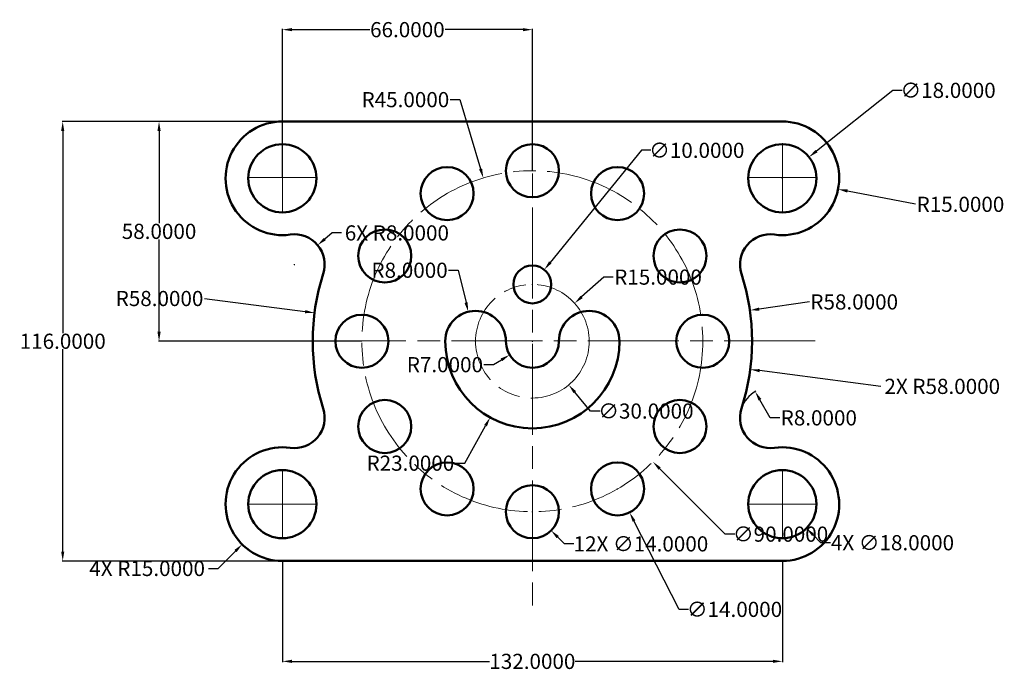
# Model space of a CAD drawing. Units: inches. Extents: x 631 to 891, y 582 to 754.
import ezdxf

# ---------------------------------------------------------------- set-up
doc = ezdxf.new("R2010")
doc.units = ezdxf.units.IN
doc.header["$MEASUREMENT"] = 0
doc.linetypes.add('ACAD_ISO08W100', pattern=[36, 24, -3, 6, -3])
for name, color, linetype, lineweight in [('M-CNTR', 4, 'ACAD_ISO08W100', 18), ('M-CNTR-MARK', 4, 'Continuous', 18), ('M-DIMS', 2, 'Continuous', 25), ('M-OUTL', 7, 'Continuous', 50)]:
    doc.layers.add(name, color=color, linetype=linetype, lineweight=lineweight)
doc.styles.get("Standard").update_dxf_attribs({"font": 'arial.ttf'})
doc.dimstyles.get("Standard").update_dxf_attribs({"dimtxt": 4, "dimasz": 2.5, "dimexe": 0.18, "dimexo": 0.0625, "dimgap": 0.09, "dimtad": 0, "dimtih": 1, "dimtoh": 1, "dimdec": 4, "dimzin": 0, "dimdsep": 46, "dimtxsty": 'Standard', "dimcen": 0.09, "dimadec": 0, "dimazin": 0, "dimtfac": 1, "dimtdec": 4, "dimtofl": 0, "dimtmove": 0, "dimatfit": 3, "dimfxl": 1, "dimtolj": 1, "dimtzin": 0, "dimarcsym": 0})

# ---------------------------------------------------------------- blocks, each defined once
blk = doc.blocks.new('*D1')
at = {"layer": 'Defpoints', "color": 0, "lineweight": 100, "transparency": 16777216}
for p in [(777.54, 678.87), (766.39, 668.84)]:
    blk.add_point(p, dxfattribs=at)
at = {"layer": 'M-DIMS', "color": 0, "lineweight": -2, "transparency": 16777216}
for p, q in [((785.22, 685.77), (779.4, 680.54)), ((787.72, 685.77), (785.22, 685.77)), ((766.3, 668.84), (766.48, 668.84)), ((766.39, 668.75), (766.39, 668.93))]:
    blk.add_line(p, q, dxfattribs=at)
at = {"layer": 'M-DIMS', "color": 0, "lineweight": 100, "transparency": 16777216}
blk.add_solid([(779.13, 680.85), (779.68, 680.23), (777.54, 678.87)], dxfattribs=at)
at = {"layer": 'M-DIMS', "color": 0, "transparency": 16777216, "insert": (799.57, 685.77), "char_height": 4, "attachment_point": 5}
blk.add_mtext('\\A1;R15.0000', dxfattribs=at)
blk = doc.blocks.new('*D2')
at = {"layer": 'Defpoints', "color": 0, "lineweight": 100, "transparency": 16777216}
for p in [(708.87, 676.33), (766.39, 668.84)]:
    blk.add_point(p, dxfattribs=at)
at = {"layer": 'M-DIMS', "color": 0, "lineweight": -2, "transparency": 16777216}
for p, q in [((679.82, 680.12), (706.39, 676.66)), ((766.3, 668.84), (766.48, 668.84)), ((766.39, 668.75), (766.39, 668.93))]:
    blk.add_line(p, q, dxfattribs=at)
at = {"layer": 'M-DIMS', "color": 0, "lineweight": 100, "transparency": 16777216}
blk.add_solid([(706.45, 677.07), (706.34, 676.24), (708.87, 676.33)], dxfattribs=at)
at = {"layer": 'M-DIMS', "color": 0, "transparency": 16777216, "insert": (667.96, 680.12), "char_height": 4, "attachment_point": 5}
blk.add_mtext('\\A1;R58.0000', dxfattribs=at)
blk = doc.blocks.new('*D3')
at = {"layer": 'Defpoints', "color": 0, "lineweight": 100, "transparency": 16777216}
for p in [(823.81, 676.99), (766.39, 668.84)]:
    blk.add_point(p, dxfattribs=at)
at = {"layer": 'M-DIMS', "color": 0, "lineweight": -2, "transparency": 16777216}
for p, q in [((839.51, 679.22), (826.29, 677.34)), ((766.3, 668.84), (766.48, 668.84)), ((766.39, 668.75), (766.39, 668.93))]:
    blk.add_line(p, q, dxfattribs=at)
at = {"layer": 'M-DIMS', "color": 0, "lineweight": 100, "transparency": 16777216}
blk.add_solid([(826.23, 677.75), (826.35, 676.93), (823.81, 676.99)], dxfattribs=at)
at = {"layer": 'M-DIMS', "color": 0, "transparency": 16777216, "insert": (851.36, 679.22), "char_height": 4, "attachment_point": 5}
blk.add_mtext('\\A1;R58.0000', dxfattribs=at)
blk = doc.blocks.new('*D4')
at = {"layer": 'Defpoints', "color": 0, "lineweight": 100, "transparency": 16777216}
for p in [(832.39, 711.84), (847.11, 708.97)]:
    blk.add_point(p, dxfattribs=at)
at = {"layer": 'M-DIMS', "color": 0, "lineweight": -2, "transparency": 16777216}
for p, q in [((832.3, 711.84), (832.48, 711.84)), ((832.39, 711.75), (832.39, 711.93)), ((867.55, 704.98), (849.56, 708.49))]:
    blk.add_line(p, q, dxfattribs=at)
at = {"layer": 'M-DIMS', "color": 0, "lineweight": 100, "transparency": 16777216}
blk.add_solid([(849.64, 708.9), (849.48, 708.08), (847.11, 708.97)], dxfattribs=at)
at = {"layer": 'M-DIMS', "color": 0, "transparency": 16777216, "insert": (879.41, 704.98), "char_height": 4, "attachment_point": 5}
blk.add_mtext('\\A1;R15.0000', dxfattribs=at)
blk = doc.blocks.new('*D5')
at = {"layer": 'Defpoints', "color": 0, "lineweight": 100, "transparency": 16777216}
for p in [(825.21, 655.55), (829.21, 648.62)]:
    blk.add_point(p, dxfattribs=at)
at = {"layer": 'M-DIMS', "color": 0, "lineweight": -2, "transparency": 16777216}
for p, q in [((829.21, 648.62), (826.46, 653.39)), ((831.71, 648.62), (829.21, 648.62))]:
    blk.add_line(p, q, dxfattribs=at)
blk.add_arc((829.21, 648.62), 8, 118.7108, 161.7121, dxfattribs=at)
at = {"layer": 'M-DIMS', "color": 0, "lineweight": 100, "transparency": 16777216}
blk.add_solid([(826.83, 653.6), (826.1, 653.18), (825.21, 655.55)], dxfattribs=at)
at = {"layer": 'M-DIMS', "color": 0, "transparency": 16777216, "insert": (842.01, 648.62), "char_height": 4, "attachment_point": 5}
blk.add_mtext('\\A1;R8.0000', dxfattribs=at)
blk = doc.blocks.new('*D6')
at = {"layer": 'Defpoints', "color": 0, "lineweight": 100, "transparency": 16777216}
for p in [(749.47, 676.61), (751.39, 668.84)]:
    blk.add_point(p, dxfattribs=at)
at = {"layer": 'M-DIMS', "color": 0, "lineweight": -2, "transparency": 16777216}
for p, q in [((744.27, 687.58), (746.77, 687.58)), ((746.77, 687.58), (748.87, 679.04)), ((751.3, 668.84), (751.48, 668.84)), ((751.39, 668.75), (751.39, 668.93))]:
    blk.add_line(p, q, dxfattribs=at)
at = {"layer": 'M-DIMS', "color": 0, "lineweight": 100, "transparency": 16777216}
blk.add_solid([(749.28, 679.14), (748.47, 678.94), (749.47, 676.61)], dxfattribs=at)
at = {"layer": 'M-DIMS', "color": 0, "transparency": 16777216, "insert": (733.97, 687.58), "char_height": 4, "attachment_point": 5}
blk.add_mtext('\\A1;R8.0000', dxfattribs=at)
blk = doc.blocks.new('*D7')
at = {"layer": 'Defpoints', "color": 0, "lineweight": 100, "transparency": 16777216}
for p in [(753.44, 711.94), (766.39, 668.84)]:
    blk.add_point(p, dxfattribs=at)
at = {"layer": 'M-DIMS', "color": 0, "lineweight": -2, "transparency": 16777216}
for p, q in [((744.73, 732.61), (747.23, 732.61)), ((747.23, 732.61), (752.72, 714.33)), ((766.3, 668.84), (766.48, 668.84)), ((766.39, 668.75), (766.39, 668.93))]:
    blk.add_line(p, q, dxfattribs=at)
at = {"layer": 'M-DIMS', "color": 0, "lineweight": 100, "transparency": 16777216}
blk.add_solid([(753.12, 714.45), (752.32, 714.21), (753.44, 711.94)], dxfattribs=at)
at = {"layer": 'M-DIMS', "color": 0, "transparency": 16777216, "insert": (732.87, 732.61), "char_height": 4, "attachment_point": 5}
blk.add_mtext('\\A1;R45.0000', dxfattribs=at)
blk = doc.blocks.new('*D8')
at = {"layer": 'Defpoints', "color": 0, "lineweight": 100, "transparency": 16777216}
for p in [(785.7, 636.11), (792.07, 623.64)]:
    blk.add_point(p, dxfattribs=at)
at = {"layer": 'M-DIMS', "color": 0, "lineweight": -2, "transparency": 16777216}
for p, q in [((788.8, 629.87), (788.98, 629.87)), ((788.89, 629.78), (788.89, 629.96)), ((805.15, 598.07), (793.21, 621.41)), ((807.65, 598.07), (805.15, 598.07))]:
    blk.add_line(p, q, dxfattribs=at)
at = {"layer": 'M-DIMS', "color": 0, "lineweight": 100, "transparency": 16777216}
blk.add_solid([(793.58, 621.6), (792.84, 621.22), (792.07, 623.64)], dxfattribs=at)
at = {"layer": 'M-DIMS', "color": 0, "transparency": 16777216, "insert": (819.76, 598.07), "char_height": 4, "attachment_point": 5}
blk.add_mtext('\\A1;∅14.0000', dxfattribs=at)
blk = doc.blocks.new('*D9')
at = {"layer": 'Defpoints', "color": 0, "lineweight": 100, "transparency": 16777216}
for p in [(769.54, 687.72), (763.23, 679.97)]:
    blk.add_point(p, dxfattribs=at)
at = {"layer": 'M-DIMS', "color": 0, "lineweight": -2, "transparency": 16777216}
for p, q in [((795.19, 719.23), (771.12, 689.66)), ((797.69, 719.23), (795.19, 719.23)), ((766.3, 683.84), (766.48, 683.84)), ((766.39, 683.75), (766.39, 683.93))]:
    blk.add_line(p, q, dxfattribs=at)
at = {"layer": 'M-DIMS', "color": 0, "lineweight": 100, "transparency": 16777216}
blk.add_solid([(770.8, 689.92), (771.45, 689.4), (769.54, 687.72)], dxfattribs=at)
at = {"layer": 'M-DIMS', "color": 0, "transparency": 16777216, "insert": (809.8, 719.23), "char_height": 4, "attachment_point": 5}
blk.add_mtext('\\A1;∅10.0000', dxfattribs=at)
blk = doc.blocks.new('*D10')
at = {"layer": 'Defpoints', "color": 0, "lineweight": 100, "transparency": 16777216}
for p in [(700.39, 610.84), (832.39, 610.84), (832.39, 584.35)]:
    blk.add_point(p, dxfattribs=at)
at = {"layer": 'M-DIMS', "color": 0, "lineweight": -2, "transparency": 16777216}
for p, q in [((700.39, 610.78), (700.39, 584.17)), ((832.39, 610.78), (832.39, 584.17)), ((702.89, 584.35), (755.08, 584.35)), ((829.89, 584.35), (777.69, 584.35))]:
    blk.add_line(p, q, dxfattribs=at)
at = {"layer": 'M-DIMS', "color": 0, "lineweight": 100, "transparency": 16777216}
for points in [[(702.89, 584.77), (702.89, 583.94), (700.39, 584.35)], [(829.89, 584.77), (829.89, 583.94), (832.39, 584.35)]]:
    blk.add_solid(points, dxfattribs=at)
at = {"layer": 'M-DIMS', "color": 0, "transparency": 16777216, "insert": (766.39, 584.35), "char_height": 4, "attachment_point": 5}
blk.add_mtext('\\A1;132.0000', dxfattribs=at)
blk = doc.blocks.new('*D11')
at = {"layer": 'Defpoints', "color": 0, "lineweight": 100, "transparency": 16777216}
for p in [(642.4, 726.84), (700.39, 726.84), (700.39, 610.84)]:
    blk.add_point(p, dxfattribs=at)
at = {"layer": 'M-DIMS', "color": 0, "lineweight": -2, "transparency": 16777216}
for p, q in [((700.33, 726.84), (642.22, 726.84)), ((642.4, 724.34), (642.4, 670.98)), ((642.4, 613.34), (642.4, 666.71)), ((700.33, 610.84), (642.22, 610.84))]:
    blk.add_line(p, q, dxfattribs=at)
at = {"layer": 'M-DIMS', "color": 0, "lineweight": 100, "transparency": 16777216}
for points in [[(641.98, 724.34), (642.81, 724.34), (642.4, 726.84)], [(641.98, 613.34), (642.81, 613.34), (642.4, 610.84)]]:
    blk.add_solid(points, dxfattribs=at)
at = {"layer": 'M-DIMS', "color": 0, "transparency": 16777216, "insert": (642.4, 668.84), "char_height": 4, "attachment_point": 5}
blk.add_mtext('\\A1;116.0000', dxfattribs=at)
blk = doc.blocks.new('*D12')
at = {"layer": 'Defpoints', "color": 0, "lineweight": 100, "transparency": 16777216}
for p in [(667.83, 726.84), (721.39, 726.84), (721.39, 668.84)]:
    blk.add_point(p, dxfattribs=at)
at = {"layer": 'M-DIMS', "color": 0, "lineweight": -2, "transparency": 16777216}
for p, q in [((721.33, 726.84), (667.65, 726.84)), ((667.83, 724.34), (667.83, 699.98)), ((667.83, 671.34), (667.83, 695.71)), ((721.33, 668.84), (667.65, 668.84))]:
    blk.add_line(p, q, dxfattribs=at)
at = {"layer": 'M-DIMS', "color": 0, "lineweight": 100, "transparency": 16777216}
for points in [[(667.41, 724.34), (668.25, 724.34), (667.83, 726.84)], [(667.41, 671.34), (668.25, 671.34), (667.83, 668.84)]]:
    blk.add_solid(points, dxfattribs=at)
at = {"layer": 'M-DIMS', "color": 0, "transparency": 16777216, "insert": (667.83, 697.84), "char_height": 4, "attachment_point": 5}
blk.add_mtext('\\A1;58.0000', dxfattribs=at)
blk = doc.blocks.new('*D13')
at = {"layer": 'Defpoints', "color": 0, "lineweight": 100, "transparency": 16777216}
for p in [(766.39, 751.08), (766.39, 713.84), (700.39, 712.08)]:
    blk.add_point(p, dxfattribs=at)
at = {"layer": 'M-DIMS', "color": 0, "lineweight": -2, "transparency": 16777216}
for p, q in [((700.39, 712.14), (700.39, 751.26)), ((766.39, 713.91), (766.39, 751.26)), ((702.89, 751.08), (723.44, 751.08)), ((763.89, 751.08), (743.34, 751.08))]:
    blk.add_line(p, q, dxfattribs=at)
at = {"layer": 'M-DIMS', "color": 0, "lineweight": 100, "transparency": 16777216}
for points in [[(702.89, 751.5), (702.89, 750.67), (700.39, 751.08)], [(763.89, 751.5), (763.89, 750.67), (766.39, 751.08)]]:
    blk.add_solid(points, dxfattribs=at)
at = {"layer": 'M-DIMS', "color": 0, "transparency": 16777216, "insert": (733.39, 751.08), "char_height": 4, "attachment_point": 5}
blk.add_mtext('\\A1;66.0000', dxfattribs=at)
blk = doc.blocks.new('*D14')
at = {"layer": 'Defpoints', "color": 0, "lineweight": 100, "transparency": 16777216}
for p in [(839.43, 717.45), (825.35, 706.23)]:
    blk.add_point(p, dxfattribs=at)
at = {"layer": 'M-DIMS', "color": 0, "lineweight": -2, "transparency": 16777216}
for p, q in [((861.52, 735.06), (841.38, 719.01)), ((864.02, 735.06), (861.52, 735.06)), ((832.3, 711.84), (832.48, 711.84)), ((832.39, 711.75), (832.39, 711.93))]:
    blk.add_line(p, q, dxfattribs=at)
at = {"layer": 'M-DIMS', "color": 0, "lineweight": 100, "transparency": 16777216}
blk.add_solid([(841.12, 719.34), (841.64, 718.69), (839.43, 717.45)], dxfattribs=at)
at = {"layer": 'M-DIMS', "color": 0, "transparency": 16777216, "insert": (876.14, 735.06), "char_height": 4, "attachment_point": 5}
blk.add_mtext('\\A1;∅18.0000', dxfattribs=at)
blk = doc.blocks.new('MOUNT-HOLE-D18')
blk.add_circle((0, 0), 9)
blk = doc.blocks.new('BOLT-CIRCLE-HOLE-D14')
blk.add_circle((0, 0), 7)
blk = doc.blocks.new('CENTER-MARK-D18')
for p, q in [((0, 9), (0, -9)), ((0, 0), (-9, 0)), ((0, 0), (9, 0))]:
    blk.add_line(p, q)
blk = doc.blocks.new('*D18')
at = {"layer": 'Defpoints', "color": 0, "lineweight": 100, "transparency": 16777216}
for p in [(700.39, 625.84), (689.78, 615.24)]:
    blk.add_point(p, dxfattribs=at)
at = {"layer": 'M-DIMS', "color": 0, "lineweight": -2, "transparency": 16777216}
for p, q in [((700.3, 625.84), (700.48, 625.84)), ((700.39, 625.75), (700.39, 625.93)), ((683.42, 608.87), (688.01, 613.47)), ((680.92, 608.87), (683.42, 608.87))]:
    blk.add_line(p, q, dxfattribs=at)
at = {"layer": 'M-DIMS', "color": 0, "lineweight": 100, "transparency": 16777216}
blk.add_solid([(687.72, 613.76), (688.31, 613.18), (689.78, 615.24)], dxfattribs=at)
at = {"layer": 'M-DIMS', "color": 0, "transparency": 16777216, "insert": (664.69, 608.87), "char_height": 4, "attachment_point": 5}
blk.add_mtext('\\A1;4X R15.0000', dxfattribs=at)
blk = doc.blocks.new('*D19')
at = {"layer": 'Defpoints', "color": 0, "lineweight": 100, "transparency": 16777216}
for p in [(766.39, 668.84), (823.91, 661.4)]:
    blk.add_point(p, dxfattribs=at)
at = {"layer": 'M-DIMS', "color": 0, "lineweight": -2, "transparency": 16777216}
for p, q in [((766.3, 668.84), (766.48, 668.84)), ((766.39, 668.75), (766.39, 668.93)), ((858.42, 656.93), (826.39, 661.08))]:
    blk.add_line(p, q, dxfattribs=at)
at = {"layer": 'M-DIMS', "color": 0, "lineweight": 100, "transparency": 16777216}
blk.add_solid([(826.44, 661.49), (826.33, 660.66), (823.91, 661.4)], dxfattribs=at)
at = {"layer": 'M-DIMS', "color": 0, "transparency": 16777216, "insert": (874.61, 656.93), "char_height": 4, "attachment_point": 5}
blk.add_mtext('\\A1;2X R58.0000', dxfattribs=at)
blk = doc.blocks.new('*D20')
at = {"layer": 'Defpoints', "color": 0, "lineweight": 100, "transparency": 16777216}
for p in [(709.69, 694.21), (703.56, 689.06)]:
    blk.add_point(p, dxfattribs=at)
at = {"layer": 'M-DIMS', "color": 0, "lineweight": -2, "transparency": 16777216}
for p, q in [((713.51, 697.43), (711.6, 695.82)), ((716.01, 697.43), (713.51, 697.43)), ((703.47, 689.06), (703.65, 689.06)), ((703.56, 688.97), (703.56, 689.15))]:
    blk.add_line(p, q, dxfattribs=at)
at = {"layer": 'M-DIMS', "color": 0, "lineweight": 100, "transparency": 16777216}
blk.add_solid([(711.33, 696.14), (711.87, 695.5), (709.69, 694.21)], dxfattribs=at)
at = {"layer": 'M-DIMS', "color": 0, "transparency": 16777216, "insert": (730.62, 697.43), "char_height": 4, "attachment_point": 5}
blk.add_mtext('\\A1;6X R8.0000', dxfattribs=at)
blk = doc.blocks.new('*D21')
at = {"layer": 'Defpoints', "color": 0, "lineweight": 100, "transparency": 16777216}
for p in [(734.57, 700.66), (798.21, 637.02)]:
    blk.add_point(p, dxfattribs=at)
at = {"layer": 'M-DIMS', "color": 0, "lineweight": -2, "transparency": 16777216}
for p, q in [((766.3, 668.84), (766.48, 668.84)), ((766.39, 668.75), (766.39, 668.93)), ((817.3, 617.93), (799.98, 635.26)), ((819.8, 617.93), (817.3, 617.93))]:
    blk.add_line(p, q, dxfattribs=at)
at = {"layer": 'M-DIMS', "color": 0, "lineweight": 100, "transparency": 16777216}
blk.add_solid([(800.27, 635.55), (799.68, 634.96), (798.21, 637.02)], dxfattribs=at)
at = {"layer": 'M-DIMS', "color": 0, "transparency": 16777216, "insert": (831.92, 617.93), "char_height": 4, "attachment_point": 5}
blk.add_mtext('\\A1;∅90.0000', dxfattribs=at)
blk = doc.blocks.new('*D22')
at = {"layer": 'Defpoints', "color": 0, "lineweight": 100, "transparency": 16777216}
for p in [(826.02, 632.21), (838.75, 619.48)]:
    blk.add_point(p, dxfattribs=at)
at = {"layer": 'M-DIMS', "color": 0, "lineweight": -2, "transparency": 16777216}
for p, q in [((832.3, 625.84), (832.48, 625.84)), ((832.39, 625.75), (832.39, 625.93)), ((842.57, 615.66), (840.52, 617.71)), ((845.07, 615.66), (842.57, 615.66))]:
    blk.add_line(p, q, dxfattribs=at)
at = {"layer": 'M-DIMS', "color": 0, "lineweight": 100, "transparency": 16777216}
blk.add_solid([(840.81, 618.01), (840.23, 617.42), (838.75, 619.48)], dxfattribs=at)
at = {"layer": 'M-DIMS', "color": 0, "transparency": 16777216, "insert": (861.46, 615.66), "char_height": 4, "attachment_point": 5}
blk.add_mtext('\\A1;4X ∅18.0000', dxfattribs=at)
blk = doc.blocks.new('*D23')
at = {"layer": 'Defpoints', "color": 0, "lineweight": 100, "transparency": 16777216}
for p in [(761.44, 628.79), (771.34, 618.89)]:
    blk.add_point(p, dxfattribs=at)
at = {"layer": 'M-DIMS', "color": 0, "lineweight": -2, "transparency": 16777216}
for p, q in [((766.39, 623.75), (766.39, 623.93)), ((766.3, 623.84), (766.48, 623.84)), ((774.87, 615.36), (773.11, 617.13)), ((777.37, 615.36), (774.87, 615.36))]:
    blk.add_line(p, q, dxfattribs=at)
at = {"layer": 'M-DIMS', "color": 0, "lineweight": 100, "transparency": 16777216}
blk.add_solid([(773.4, 617.42), (772.81, 616.83), (771.34, 618.89)], dxfattribs=at)
at = {"layer": 'M-DIMS', "color": 0, "transparency": 16777216, "insert": (795.05, 615.36), "char_height": 4, "attachment_point": 5}
blk.add_mtext('\\A1;12X ∅14.0000', dxfattribs=at)
blk = doc.blocks.new('*D24')
at = {"layer": 'Defpoints', "color": 0, "lineweight": 100, "transparency": 16777216}
for p in [(766.39, 668.84), (755.24, 648.73)]:
    blk.add_point(p, dxfattribs=at)
at = {"layer": 'M-DIMS', "color": 0, "lineweight": -2, "transparency": 16777216}
for p, q in [((766.3, 668.84), (766.48, 668.84)), ((766.39, 668.75), (766.39, 668.93)), ((748.55, 636.66), (754.03, 646.54)), ((746.05, 636.66), (748.55, 636.66))]:
    blk.add_line(p, q, dxfattribs=at)
at = {"layer": 'M-DIMS', "color": 0, "lineweight": 100, "transparency": 16777216}
blk.add_solid([(753.66, 646.74), (754.39, 646.34), (755.24, 648.73)], dxfattribs=at)
at = {"layer": 'M-DIMS', "color": 0, "transparency": 16777216, "insert": (734.19, 636.66), "char_height": 4, "attachment_point": 5}
blk.add_mtext('\\A1;R23.0000', dxfattribs=at)
blk = doc.blocks.new('*D25')
at = {"layer": 'Defpoints', "color": 0, "lineweight": 100, "transparency": 16777216}
for p in [(766.39, 668.84), (760.39, 665.24)]:
    blk.add_point(p, dxfattribs=at)
at = {"layer": 'M-DIMS', "color": 0, "lineweight": -2, "transparency": 16777216}
for p, q in [((766.3, 668.84), (766.48, 668.84)), ((766.39, 668.75), (766.39, 668.93)), ((756.1, 662.66), (758.25, 663.95)), ((753.6, 662.66), (756.1, 662.66))]:
    blk.add_line(p, q, dxfattribs=at)
at = {"layer": 'M-DIMS', "color": 0, "lineweight": 100, "transparency": 16777216}
blk.add_solid([(758.03, 664.31), (758.46, 663.59), (760.39, 665.24)], dxfattribs=at)
at = {"layer": 'M-DIMS', "color": 0, "transparency": 16777216, "insert": (743.3, 662.66), "char_height": 4, "attachment_point": 5}
blk.add_mtext('\\A1;R7.0000', dxfattribs=at)
blk = doc.blocks.new('*D26')
at = {"layer": 'Defpoints', "color": 0, "lineweight": 100, "transparency": 16777216}
for p in [(756.79, 680.37), (775.99, 657.32)]:
    blk.add_point(p, dxfattribs=at)
at = {"layer": 'M-DIMS', "color": 0, "lineweight": -2, "transparency": 16777216}
for p, q in [((766.3, 668.84), (766.48, 668.84)), ((766.39, 668.75), (766.39, 668.93)), ((781.75, 650.41), (777.59, 655.4)), ((784.25, 650.41), (781.75, 650.41))]:
    blk.add_line(p, q, dxfattribs=at)
at = {"layer": 'M-DIMS', "color": 0, "lineweight": 100, "transparency": 16777216}
blk.add_solid([(777.91, 655.67), (777.27, 655.13), (775.99, 657.32)], dxfattribs=at)
at = {"layer": 'M-DIMS', "color": 0, "transparency": 16777216, "insert": (796.37, 650.41), "char_height": 4, "attachment_point": 5}
blk.add_mtext('\\A1;∅30.0000', dxfattribs=at)

msp = doc.modelspace()

# ---------------------------------------------------------------- linework, layer by layer
at = {"layer": 'M-CNTR'}
for p, q in [((766.38827, 740.12463), (766.38827, 597.79966)), ((841.02678, 668.96214), (692.87285, 668.96214))]:
    msp.add_line(p, q, dxfattribs=at)
for radius in [45, 15]:
    msp.add_circle((766.38827, 668.84399), radius, dxfattribs=at)
at = {"layer": 'M-OUTL'}
for p, q in [((700.38827, 726.84399), (832.38827, 726.84399)), ((700.38827, 610.84399), (832.38827, 610.84399))]:
    msp.add_line(p, q, dxfattribs=at)
msp.add_circle((766.38827, 683.84399), 5, dxfattribs=at)
for centre, radius, start, end in [((700.38827, 711.84399), 15, 90, 277.9312313), ((832.38827, 711.84399), 15, 262.0687687, 90), ((703.56191, 689.064), 8, 342.1597695, 97.9312313), ((829.21463, 689.064), 8, 82.0687687, 197.8402305), ((766.38827, 668.84399), 58, 162.1597695, 197.8402305), ((766.38827, 668.84399), 58, 342.1597695, 17.8402305), ((751.38827, 668.84399), 8, 0, 180), ((781.38827, 668.84399), 8, 0, 180), ((766.38827, 668.84399), 23, 180, 0), ((766.38827, 668.84399), 7, 180, 0), ((703.56191, 648.62398), 8, 262.0687687, 17.8402305), ((829.21463, 648.62398), 8, 162.1597695, 277.9312313), ((700.38827, 625.84399), 15, 82.0687687, 270), ((832.38827, 625.84399), 15, 270, 97.9312313)]:
    msp.add_arc(centre, radius, start, end, dxfattribs=at)

# ---------------------------------------------------------------- block references
at = {"layer": 'M-CNTR-MARK'}
for p in [(700.38827, 712.08029), (832.38827, 712.08029), (832.38827, 625.84399)]:
    msp.add_blockref('CENTER-MARK-D18', p, dxfattribs=at)
at = {"layer": 'M-CNTR-MARK', "rotation": 180}
msp.add_blockref('CENTER-MARK-D18', (700.38827, 625.84399), dxfattribs=at)
at = {"layer": 'M-OUTL'}
for name, p in [('MOUNT-HOLE-D18', (700.38827, 711.84399)), ('BOLT-CIRCLE-HOLE-D14', (766.38827, 713.84399)), ('MOUNT-HOLE-D18', (832.38827, 711.84399)), ('BOLT-CIRCLE-HOLE-D14', (743.88827, 707.81514)), ('BOLT-CIRCLE-HOLE-D14', (788.88827, 707.81514)), ('BOLT-CIRCLE-HOLE-D14', (727.41713, 691.34399)), ('BOLT-CIRCLE-HOLE-D14', (805.35941, 691.34399)), ('BOLT-CIRCLE-HOLE-D14', (721.38827, 668.84399)), ('BOLT-CIRCLE-HOLE-D14', (811.38827, 668.84399)), ('BOLT-CIRCLE-HOLE-D14', (727.41713, 646.34399)), ('BOLT-CIRCLE-HOLE-D14', (805.35941, 646.34399)), ('BOLT-CIRCLE-HOLE-D14', (743.88827, 629.87285)), ('BOLT-CIRCLE-HOLE-D14', (788.88827, 629.87285)), ('MOUNT-HOLE-D18', (700.38827, 625.84399)), ('MOUNT-HOLE-D18', (832.38827, 625.84399)), ('BOLT-CIRCLE-HOLE-D14', (766.38827, 623.84399))]:
    msp.add_blockref(name, p, dxfattribs=at)

# ---------------------------------------------------------------- dimensions: what is measured, and where the dimension line sits
at = {"layer": 'M-DIMS'}
for base, p1, p2, picture, middle in [((766.38827, 751.08415), (700.38827, 712.08029), (766.38827, 713.84399), '*D13', (733.38827, 751.08415)), ((832.38827, 584.35212), (700.38827, 610.84399), (832.38827, 610.84399), '*D10', (766.38827, 584.35212))]:
    dim = msp.add_linear_dim(base=base, p1=p1, p2=p2, dimstyle='Standard', override={"dimclrd": 0, "dimclre": 0, "dimclrt": 0}, dxfattribs=at)
    dim.commit()
    dim.dimension.update_dxf_attribs({"geometry": picture, "text_midpoint": middle})
for p1, p2, override, picture, middle in [((825.34999, 706.23483), (839.42655, 717.45315), {"dimclrd": 0, "dimclre": 0, "dimclrt": 0}, '*D14', (876.13632, 735.06085)), ((763.23248, 679.96572), (769.54406, 687.72226), {"dimclrd": 0, "dimclre": 0, "dimclrt": 0}, '*D9', (809.80145, 719.23404)), ((734.5686, 700.66393), (798.20794, 637.02406), {"dimdec": 4, "dimlfac": 1, "dimrnd": 0, "dimzin": 0, "dimdsep": 46, "dimlunit": 2}, '*D21', (831.91567, 617.93209)), ((756.78645, 680.3681), (775.99009, 657.31989), {"dimdec": 4, "dimlfac": 1, "dimrnd": 0, "dimzin": 0, "dimdsep": 46, "dimlunit": 2}, '*D26', (796.36711, 650.40543)), ((785.70231, 636.1058), (792.07423, 623.6399), {"dimclrd": 0, "dimclre": 0, "dimclrt": 0}, '*D8', (819.76177, 598.06678))]:
    dim = msp.add_diameter_dim_2p(p1=p1, p2=p2, dimstyle='Standard', override=override, dxfattribs=at)
    dim.commit()
    dim.dimension.update_dxf_attribs({"geometry": picture, "text_midpoint": middle, "dimtype": 163})
for center, mpoint, override, picture, middle in [((766.38827, 668.84399), (753.43666, 711.93988), {"dimclrd": 0, "dimclre": 0, "dimclrt": 0}, '*D7', (732.87159, 732.607)), ((832.38827, 711.84399), (847.11036, 708.96994), {"dimclrd": 0, "dimclre": 0, "dimclrt": 0}, '*D4', (867.55304, 704.97911)), ((751.38827, 668.84399), (749.47252, 676.61122), {"dimclrd": 0, "dimclre": 0, "dimclrt": 0}, '*D6', (733.96763, 687.57754)), ((766.38827, 668.84399), (777.54444, 678.87095), {"dimclrd": 0, "dimclre": 0, "dimclrt": 0}, '*D1', (799.57396, 685.76958)), ((766.38827, 668.84399), (708.87405, 676.33498), {"dimclrd": 0, "dimclre": 0, "dimclrt": 0}, '*D2', (679.81556, 680.11972)), ((766.38827, 668.84399), (823.8134, 676.9898), {"dimclrd": 0, "dimclre": 0, "dimclrt": 0}, '*D3', (839.50552, 679.21575)), ((766.38827, 668.84399), (755.23849, 648.72727), {"dimdec": 4, "dimlfac": 1, "dimrnd": 0, "dimzin": 0, "dimdsep": 46, "dimlunit": 2}, '*D24', (734.19464, 636.65724)), ((829.21463, 648.62398), (825.21463, 655.55219), {"dimclrd": 0, "dimclre": 0, "dimclrt": 0}, '*D5', (842.01472, 648.62398))]:
    dim = msp.add_radius_dim(center=center, mpoint=mpoint, dimstyle='Standard', override=override, dxfattribs=at)
    dim.commit()
    dim.dimension.update_dxf_attribs({"geometry": picture, "text_midpoint": middle, "dimtype": 164})
for base, p1, p2, picture, middle in [((642.39822, 726.84399), (700.38827, 610.84399), (700.38827, 726.84399), '*D11', (642.39822, 668.84399)), ((667.83107, 726.84399), (721.38827, 668.84399), (721.38827, 726.84399), '*D12', (667.83107, 697.84399))]:
    dim = msp.add_linear_dim(base=base, p1=p1, p2=p2, angle=90, dimstyle='Standard', override={"dimclrd": 0, "dimclre": 0, "dimclrt": 0}, dxfattribs=at)
    dim.commit()
    dim.dimension.update_dxf_attribs({"geometry": picture, "text_midpoint": middle})
dim = msp.add_radius_dim(center=(703.56191, 689.064), mpoint=(709.68619, 694.21116), text='6X <>', dimstyle='Standard', override={"dimdec": 4, "dimlfac": 1, "dimrnd": 0, "dimzin": 0, "dimdsep": 46, "dimlunit": 2}, dxfattribs=at)
dim.commit()
dim.dimension.update_dxf_attribs({"geometry": '*D20', "text_midpoint": (730.62228, 697.42813)})
dim = msp.add_radius_dim(center=(766.38827, 668.84399), mpoint=(760.38804, 665.23882), dimstyle='Standard', override={"dimdec": 4, "dimlfac": 1, "dimrnd": 0, "dimzin": 0, "dimdsep": 46, "dimlunit": 2}, dxfattribs=at)
dim.commit()
dim.dimension.update_dxf_attribs({"geometry": '*D25', "text_midpoint": (743.30207, 662.6637)})
for center, mpoint, text, picture, middle in [((766.38827, 668.84399), (823.90845, 661.39891), '2X <>', '*D19', (858.42055, 656.93186)), ((700.38827, 625.84399), (689.78153, 615.23753), '4X <>', '*D18', (664.6856, 608.87365))]:
    dim = msp.add_radius_dim(center=center, mpoint=mpoint, text=text, dimstyle='Standard', override={"dimdec": 4, "dimlfac": 1, "dimrnd": 0, "dimzin": 0, "dimdsep": 46, "dimlunit": 2}, dxfattribs=at)
    dim.commit()
    dim.dimension.update_dxf_attribs({"geometry": picture, "text_midpoint": middle, "dimtype": 164})
for p1, p2, text, picture, middle in [((826.02444, 632.20808), (838.7521, 619.4799), '4X <>', '*D22', (861.45781, 615.66144)), ((761.43865, 628.79387), (771.33789, 618.89411), '12X <>', '*D23', (795.04586, 615.35849))]:
    dim = msp.add_diameter_dim_2p(p1=p1, p2=p2, text=text, dimstyle='Standard', override={"dimdec": 4, "dimlfac": 1, "dimrnd": 0, "dimzin": 0, "dimdsep": 46, "dimlunit": 2}, dxfattribs=at)
    dim.commit()
    dim.dimension.update_dxf_attribs({"geometry": picture, "text_midpoint": middle, "dimtype": 163})

doc.saveas('drawing.dxf')
